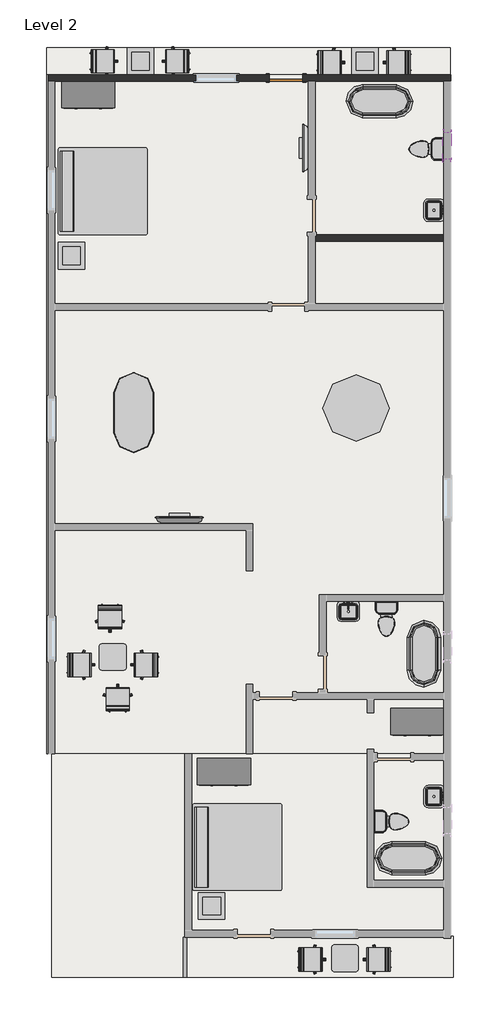
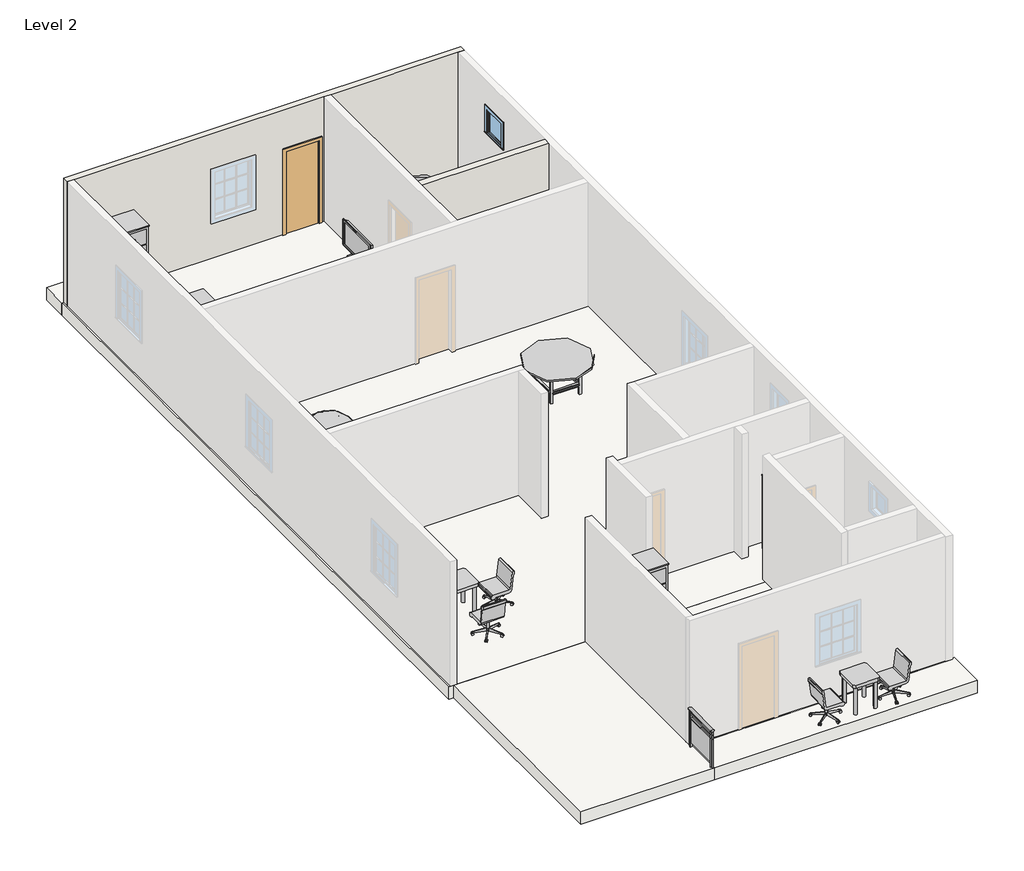
# One storey, part 2 of 2: 25 furniture elements, 9 flow terminals, 5 slabs, 2 walls, 1 door, 1 railing, 1 window.
"""IFC4 building model written with IfcOpenShell, lengths in millimetres."""

from ifc_helpers import new_model, si_unit, point, frame, origin, place, context, project, spatial, polyline, ellipse_curve, trimmed, outline, extrude, faceted_brep, transform, mapped, element, save
from ifc_brep_helpers import plane_surface, extruded_surface, advanced_brep
from components import door_255cab33, flow_terminal_62a433f7, toilet_domestic_3d_toilet_domestic_3d_f7549cf7, toilet_domestic_3d_toilet_domestic_3d_183bbd19, flow_terminal_b374fae2, furniture_1fc5af50, chair_task_chair_task_b7f3823b, furniture_9fa109b2, furniture_7a3aaa4f, furniture_b5c51a22, furniture_2c34a4f9, furniture_bbcc68ce, furniture_bcf351fa, window_3d781103

model = new_model("IFC4")

# Units and contexts
model_context = context("Model", 3, world=origin())
ifc_project = project(units=[si_unit("LENGTHUNIT", "METRE", prefix="MILLI")], contexts=[model_context])

# Site, building, storey
site = spatial("IfcSite", under=ifc_project)
building = spatial("IfcBuilding", under=site)
storey = spatial("IfcBuildingStorey", under=building, Name="Level 2", Elevation=3048.0)

# Door
placement = place(None, origin())
door_shape = door_255cab33(model_context)
element("IfcDoor", 1, ObjectType="Single-Flush : 30\" x 80\"", at=placement, inside=storey, context=model_context, shape_type="MappedRepresentation", body=[
    mapped(door_shape, transform((-7116.1873398, 12389.5549175, 3048.0), x_axis=(1.0, 0.0, 0.0), y_axis=(0.0, 1.0, 0.0), z_axis=(0.0, 0.0, 1.0))),
])

# Flow terminals
flow_terminal_shape = flow_terminal_62a433f7(model_context)
element("IfcFlowTerminal", 2, ObjectType="Sink Vanity-Square : 20\" x 18\"", at=placement, inside=storey, context=model_context, shape_type="MappedRepresentation", body=[
    mapped(flow_terminal_shape, transform((-3689.5327409, -4015.8558419, 3352.8), x_axis=(0.0, -0.9999999999999997, 0.0), y_axis=(0.9999999999999997, 0.0, 0.0), z_axis=(0.0, 0.0, 1.0))),
])
element("IfcFlowTerminal", 3, ObjectType="Sink Vanity-Square : 20\" x 18\"", at=placement, inside=storey, context=model_context, shape_type="MappedRepresentation", body=[
    mapped(flow_terminal_shape, transform((-5709.4765804, 246.0095164, 3048.0), x_axis=(1.0, 0.0, 0.0), y_axis=(0.0, 1.0, 0.0), z_axis=(0.0, 0.0, 1.0))),
])
element("IfcFlowTerminal", 4, ObjectType="Sink Vanity-Square : 20\" x 18\"", at=placement, inside=storey, context=model_context, shape_type="MappedRepresentation", body=[
    mapped(flow_terminal_shape, transform((-3689.5327409, 9382.6441581, 3352.8), x_axis=(0.0, -1.0000000000000004, 0.0), y_axis=(1.0000000000000004, 0.0, 0.0), z_axis=(0.0, 0.0, 1.0))),
])
toilet_domestic_3d_toilet_domestic_3d_shape = toilet_domestic_3d_toilet_domestic_3d_f7549cf7(model_context)
toilet_domestic_3d_toilet_domestic_3d_2_shape = toilet_domestic_3d_toilet_domestic_3d_183bbd19(model_context)
element("IfcFlowTerminal", 5, ObjectType="Toilet-Domestic-3D : Toilet-Domestic-3D", at=placement, inside=storey, context=model_context, shape_type="MappedRepresentation", body=[
    mapped(toilet_domestic_3d_toilet_domestic_3d_shape, transform((-4004.0833671, 10763.9549175, 3048.0), x_axis=(0.0, -1.0000000000000004, 0.0), y_axis=(1.0000000000000004, 0.0, 0.0), z_axis=(0.0, 0.0, 1.0))),
    mapped(toilet_domestic_3d_toilet_domestic_3d_2_shape, transform((-4004.0833671, 10763.9549175, 3048.0), x_axis=(0.0, -1.0000000000000004, 0.0), y_axis=(1.0000000000000004, 0.0, 0.0), z_axis=(0.0, 0.0, 1.0))),
])
element("IfcFlowTerminal", 6, ObjectType="Toilet-Domestic-3D : Toilet-Domestic-3D", at=placement, inside=storey, context=model_context, shape_type="MappedRepresentation", body=[
    mapped(toilet_domestic_3d_toilet_domestic_3d_shape, transform((-4614.8913124, -4603.0450825, 3048.0), x_axis=(0.0, 1.0, 0.0), y_axis=(-1.0, 0.0, 0.0), z_axis=(0.0, 0.0, 1.0))),
    mapped(toilet_domestic_3d_toilet_domestic_3d_2_shape, transform((-4614.8913124, -4603.0450825, 3048.0), x_axis=(0.0, 1.0, 0.0), y_axis=(-1.0, 0.0, 0.0), z_axis=(0.0, 0.0, 1.0))),
])
element("IfcFlowTerminal", 7, ObjectType="Toilet-Domestic-3D : Toilet-Domestic-3D", at=placement, inside=storey, context=model_context, shape_type="MappedRepresentation", body=[
    mapped(toilet_domestic_3d_toilet_domestic_3d_shape, transform((-4823.8668352, -68.5411098, 3048.0), x_axis=(1.0, 0.0, 0.0), y_axis=(0.0, 1.0, 0.0), z_axis=(0.0, 0.0, 1.0))),
    mapped(toilet_domestic_3d_toilet_domestic_3d_2_shape, transform((-4823.8668352, -68.5411098, 3048.0), x_axis=(1.0, 0.0, 0.0), y_axis=(0.0, 1.0, 0.0), z_axis=(0.0, 0.0, 1.0))),
])
flow_terminal_2_shape = flow_terminal_b374fae2(model_context)
element("IfcFlowTerminal", 8, ObjectType="Tub-Free Standing-3D : 30\" x 60\"", at=placement, inside=storey, context=model_context, shape_type="MappedRepresentation", body=[
    mapped(flow_terminal_2_shape, transform((-4322.1873398, -5441.2450825, 3048.0), x_axis=(0.0, -0.9999999999999998, 0.0), y_axis=(0.9999999999999998, 0.0, 0.0), z_axis=(0.0, 0.0, 1.0))),
])
element("IfcFlowTerminal", 9, ObjectType="Tub-Free Standing-3D : 30\" x 60\"", at=placement, inside=storey, context=model_context, shape_type="MappedRepresentation", body=[
    mapped(flow_terminal_2_shape, transform((-3966.5873398, -767.6450825, 3048.0), x_axis=(1.0, 0.0, 0.0), y_axis=(0.0, 1.0, 0.0), z_axis=(0.0, 0.0, 1.0))),
])
element("IfcFlowTerminal", 10, ObjectType="Tub-Free Standing-3D : 30\" x 60\"", at=placement, inside=storey, context=model_context, shape_type="MappedRepresentation", body=[
    mapped(flow_terminal_2_shape, transform((-4982.5873398, 11856.1549175, 3048.0), x_axis=(0.0, 1.0, 0.0), y_axis=(-1.0, 0.0, 0.0), z_axis=(0.0, 0.0, 1.0))),
])

# Furniture
furniture_shape = furniture_1fc5af50(model_context)
element("IfcFurniture", 11, ObjectType="Bed-Standard : King 78\" x 80\"", at=placement, inside=storey, context=model_context, shape_type="MappedRepresentation", body=[
    mapped(furniture_shape, transform((-8279.3824218, -5458.733607, 3048.0), x_axis=(0.0, 1.0000000000000002, 0.0), y_axis=(-1.0000000000000002, 0.0, 0.0), z_axis=(0.0, 0.0, 1.0))),
])
element("IfcFurniture", 12, ObjectType="Bed-Standard : King 78\" x 80\"", at=placement, inside=storey, context=model_context, shape_type="MappedRepresentation", body=[
    mapped(furniture_shape, transform((-11352.7824218, 9527.266393, 3048.0), x_axis=(0.0, 1.0000000000000002, 0.0), y_axis=(-1.0000000000000002, 0.0, 0.0), z_axis=(0.0, 0.0, 1.0))),
])
chair_task_chair_task_shape = chair_task_chair_task_b7f3823b(model_context)
element("IfcFurniture", 13, ObjectType="Chair-Task : Chair-Task", at=placement, inside=storey, context=model_context, shape_type="MappedRepresentation", body=[
    mapped(chair_task_chair_task_shape, transform((-9586.4414382, 12629.5640979, 3048.0), x_axis=(0.0, 1.0000000000000009, 0.0), y_axis=(-1.0000000000000009, 0.0, 0.0), z_axis=(0.0, 0.0, 1.0))),
])
element("IfcFurniture", 14, ObjectType="Chair-Task : Chair-Task", at=placement, inside=storey, context=model_context, shape_type="MappedRepresentation", body=[
    mapped(chair_task_chair_task_shape, transform((-6144.5332414, 12886.1457372, 3048.0), x_axis=(0.0, -1.0000000000000007, 0.0), y_axis=(1.0000000000000007, 0.0, 0.0), z_axis=(0.0, 0.0, 1.0))),
])
element("IfcFurniture", 15, ObjectType="Chair-Task : Chair-Task", at=placement, inside=storey, context=model_context, shape_type="MappedRepresentation", body=[
    mapped(chair_task_chair_task_shape, transform((-4531.8414382, 12604.1640979, 3048.0), x_axis=(0.0, 1.0000000000000007, 0.0), y_axis=(-1.0000000000000007, 0.0, 0.0), z_axis=(0.0, 0.0, 1.0))),
])
element("IfcFurniture", 16, ObjectType="Chair-Task : Chair-Task", at=placement, inside=storey, context=model_context, shape_type="MappedRepresentation", body=[
    mapped(chair_task_chair_task_shape, transform((-11326.1332414, 12911.5457372, 3048.0), x_axis=(0.0, -1.0000000000000009, 0.0), y_axis=(1.0000000000000009, 0.0, 0.0), z_axis=(0.0, 0.0, 1.0))),
])
element("IfcFurniture", 17, ObjectType="Chair-Task : Chair-Task", at=placement, inside=storey, context=model_context, shape_type="MappedRepresentation", body=[
    mapped(chair_task_chair_task_shape, transform((-4989.0414382, -7893.6359021, 3048.0), x_axis=(0.0, 1.0000000000000009, 0.0), y_axis=(-1.0000000000000009, 0.0, 0.0), z_axis=(0.0, 0.0, 1.0))),
])
element("IfcFurniture", 18, ObjectType="Chair-Task : Chair-Task", at=placement, inside=storey, context=model_context, shape_type="MappedRepresentation", body=[
    mapped(chair_task_chair_task_shape, transform((-6576.3332414, -7611.6542628, 3048.0), x_axis=(0.0, -1.0000000000000004, 0.0), y_axis=(1.0000000000000004, 0.0, 0.0), z_axis=(0.0, 0.0, 1.0))),
])
element("IfcFurniture", 19, ObjectType="Chair-Task : Chair-Task", at=placement, inside=storey, context=model_context, shape_type="MappedRepresentation", body=[
    mapped(chair_task_chair_task_shape, transform((-11105.2781595, -1827.9909841, 3048.0), x_axis=(1.0, 0.0, 0.0), y_axis=(0.0, 1.0, 0.0), z_axis=(0.0, 0.0, 1.0))),
])
element("IfcFurniture", 20, ObjectType="Chair-Task : Chair-Task", at=placement, inside=storey, context=model_context, shape_type="MappedRepresentation", body=[
    mapped(chair_task_chair_task_shape, transform((-11001.0965201, 89.5008192, 3048.0), x_axis=(-1.0000000000000004, 0.0, 0.0), y_axis=(0.0, -1.0000000000000004, 0.0), z_axis=(0.0, 0.0, 1.0))),
])
element("IfcFurniture", 21, ObjectType="Chair-Task : Chair-Task", at=placement, inside=storey, context=model_context, shape_type="MappedRepresentation", body=[
    mapped(chair_task_chair_task_shape, transform((-10297.6414382, -1162.6359021, 3048.0), x_axis=(0.0, 1.000000000000001, 0.0), y_axis=(-1.000000000000001, 0.0, 0.0), z_axis=(0.0, 0.0, 1.0))),
])
element("IfcFurniture", 22, ObjectType="Chair-Task : Chair-Task", at=placement, inside=storey, context=model_context, shape_type="MappedRepresentation", body=[
    mapped(chair_task_chair_task_shape, transform((-11853.1832414, -880.6542628, 3048.0), x_axis=(0.0, -1.0000000000000007, 0.0), y_axis=(1.0000000000000007, 0.0, 0.0), z_axis=(0.0, 0.0, 1.0))),
])
furniture_2_shape = furniture_9fa109b2(model_context)
element("IfcFurniture", 23, ObjectType="Dresser : 48\" x 72\" x 24\"", at=placement, inside=storey, context=model_context, shape_type="MappedRepresentation", body=[
    mapped(furniture_2_shape, transform((-8269.39408, -3096.8821284, 3048.0), x_axis=(1.0, 0.0, 0.0), y_axis=(0.0, 1.0, 0.0), z_axis=(0.0, 0.0, 1.0))),
])
element("IfcFurniture", 24, ObjectType="Dresser : 48\" x 72\" x 24\"", at=placement, inside=storey, context=model_context, shape_type="MappedRepresentation", body=[
    mapped(furniture_2_shape, transform((-11368.19408, 12371.7178716, 3048.0), x_axis=(1.0, 0.0, 0.0), y_axis=(0.0, 1.0, 0.0), z_axis=(0.0, 0.0, 1.0))),
])
element("IfcFurniture", 25, ObjectType="Dresser : 48\" x 72\" x 24\"", at=placement, inside=storey, context=model_context, shape_type="MappedRepresentation", body=[
    mapped(furniture_2_shape, transform((-3849.79408, -1953.8821284, 3048.0), x_axis=(1.0, 0.0, 0.0), y_axis=(0.0, 1.0, 0.0), z_axis=(0.0, 0.0, 1.0))),
])
furniture_3_shape = furniture_7a3aaa4f(model_context)
element("IfcFurniture", 26, ObjectType="TV - Flat Screen : 42\"", at=placement, inside=storey, context=model_context, shape_type="MappedRepresentation", body=[
    mapped(furniture_3_shape, transform((-6666.7259634, 10785.4104034, 3048.0), x_axis=(0.0, -1.0000000000000002, 0.0), y_axis=(1.0000000000000002, 0.0, 0.0), z_axis=(0.0, 0.0, 1.0))),
])
element("IfcFurniture", 27, ObjectType="TV - Flat Screen : 42\"", at=placement, inside=storey, context=model_context, shape_type="MappedRepresentation", body=[
    mapped(furniture_3_shape, transform((-9558.5318539, 2288.0935412, 3962.4), x_axis=(-1.000000000000001, 0.0, 0.0), y_axis=(0.0, -1.000000000000001, 0.0), z_axis=(0.0, 0.0, 1.0))),
])
furniture_4_shape = furniture_b5c51a22(model_context)
element("IfcFurniture", 28, ObjectType="Table-Coffee : 24\" x 24\" x 24\"", at=placement, inside=storey, context=model_context, shape_type="MappedRepresentation", body=[
    mapped(furniture_4_shape, transform((-10461.8531065, 12675.3438397, 3048.0), x_axis=(1.0, 0.0, 0.0), y_axis=(0.0, 1.0, 0.0), z_axis=(0.0, 0.0, 1.0))),
])
element("IfcFurniture", 29, ObjectType="Table-Coffee : 24\" x 24\" x 24\"", at=placement, inside=storey, context=model_context, shape_type="MappedRepresentation", body=[
    mapped(furniture_4_shape, transform((-5331.0531065, 12675.3438397, 3048.0), x_axis=(1.0, 0.0, 0.0), y_axis=(0.0, 1.0, 0.0), z_axis=(0.0, 0.0, 1.0))),
])
element("IfcFurniture", 30, ObjectType="Table-Coffee : 24\" x 24\" x 24\"", at=placement, inside=storey, context=model_context, shape_type="MappedRepresentation", body=[
    mapped(furniture_4_shape, transform((-8836.2531065, -6628.6561603, 3048.0), x_axis=(1.0, 0.0, 0.0), y_axis=(0.0, 1.0, 0.0), z_axis=(0.0, 0.0, 1.0))),
])
element("IfcFurniture", 31, ObjectType="Table-Coffee : 24\" x 24\" x 24\"", at=placement, inside=storey, context=model_context, shape_type="MappedRepresentation", body=[
    mapped(furniture_4_shape, transform((-12036.6531065, 8230.3438397, 3048.0), x_axis=(1.0, 0.0, 0.0), y_axis=(0.0, 1.0, 0.0), z_axis=(0.0, 0.0, 1.0))),
])
furniture_5_shape = furniture_2c34a4f9(model_context)
element("IfcFurniture", 32, ObjectType="Table-Dining Oval : 36\" x 72\"", at=placement, inside=storey, context=model_context, shape_type="MappedRepresentation", body=[
    mapped(furniture_5_shape, transform((-10954.0857004, 5145.9745897, 3048.0), x_axis=(0.0, 1.0000000000000002, 0.0), y_axis=(-1.0000000000000002, 0.0, 0.0), z_axis=(0.0, 0.0, 1.0))),
])
furniture_6_shape = furniture_bbcc68ce(model_context)
element("IfcFurniture", 33, ObjectType="Table-Dining Round w Chairs : 60\" Diameter", at=placement, inside=storey, context=model_context, shape_type="MappedRepresentation", body=[
    mapped(furniture_6_shape, transform((-5619.669307, 5030.6336061, 3048.0), x_axis=(1.0, 0.0, 0.0), y_axis=(0.0, 1.0, 0.0), z_axis=(0.0, 0.0, 1.0))),
])
furniture_7_shape = furniture_bcf351fa(model_context)
element("IfcFurniture", 34, ObjectType="Table-End : 24\" x 24\"", at=placement, inside=storey, context=model_context, shape_type="MappedRepresentation", body=[
    mapped(furniture_7_shape, transform((-6078.5209701, -7879.6450825, 3048.0), x_axis=(1.0, 0.0, 0.0), y_axis=(0.0, 1.0, 0.0), z_axis=(0.0, 0.0, 1.0))),
])
element("IfcFurniture", 35, ObjectType="Table-End : 24\" x 24\"", at=placement, inside=storey, context=model_context, shape_type="MappedRepresentation", body=[
    mapped(furniture_7_shape, transform((-11387.1209701, -996.2450825, 3048.0), x_axis=(1.0, 0.0, 0.0), y_axis=(0.0, 1.0, 0.0), z_axis=(0.0, 0.0, 1.0))),
])

# Railing
element("IfcRailing", 36, ObjectType="Glass Panel - Bottom Fill", at=placement, inside=storey, context=model_context, shape_type="SolidModel", body=[
    advanced_brep(
    [(-9389.4873398, -7244.6450825, 3962.4), (-9465.6873398, -7244.6450825, 3962.4), (-9389.4873398, -8159.0450825, 3962.4), (-9465.6873398, -8159.0450825, 3962.4)],
    [
        (0, 1, ellipse_curve(frame((-9427.5873398, -7244.6450825, 3962.4), z_axis=(0.0, 1.0, 0.0), x_axis=(-1.0, 0.0, 0.0)), 38.1, 28.575)),
        (1, 0, ellipse_curve(frame((-9427.5873398, -7244.6450825, 3962.4), z_axis=(0.0, 1.0, 0.0), x_axis=(-1.0, 0.0, 0.0)), 38.1, 28.575)),
        (2, 3, ellipse_curve(frame((-9427.5873398, -8159.0450825, 3962.4), z_axis=(0.0, -1.0, 0.0), x_axis=(-1.0, 0.0, 0.0)), 38.1, 28.575)),
        (3, 2, ellipse_curve(frame((-9427.5873398, -8159.0450825, 3962.4), z_axis=(0.0, -1.0, 0.0), x_axis=(-1.0, 0.0, 0.0)), 38.1, 28.575)),
        (0, 2),
        (3, 1),
    ],
    [
        plane_surface(frame((-9427.5873398, -7244.6450825, 3962.4), z_axis=(0.0, 1.0, 0.0), x_axis=(0.0, 0.0, -1.0))),
        plane_surface(frame((-9427.5873398, -8159.0450825, 3962.4), z_axis=(0.0, -1.0, 0.0), x_axis=(0.0, 0.0, -1.0))),
        extruded_surface(trimmed(ellipse_curve(frame((-9427.5873398, -8159.0450825, 3962.4), z_axis=(0.0, 1.0, 0.0), x_axis=(-1.0, 0.0, 0.0)), 38.1, 28.575), [point((-9389.4873398, -8159.0450825, 3962.4))], [point((-9465.6873398, -8159.0450825, 3962.4))], True, "CARTESIAN"), (0.0, 914.3999999999996, 0.0), 914.3999999999996),
        extruded_surface(trimmed(ellipse_curve(frame((-9427.5873398, -8159.0450825, 3962.4), z_axis=(0.0, 1.0, 0.0), x_axis=(-1.0, 0.0, 0.0)), 38.1, 28.575), [point((-9465.6873398, -8159.0450825, 3962.4))], [point((-9389.4873398, -8159.0450825, 3962.4))], True, "CARTESIAN"), (0.0, 914.3999999999996, 0.0), 914.3999999999996),
    ],
    [
        (0, [[1, 2]]),
        (1, [[3, 4]]),
        (2, [[-1, 5, -4, 6]]),
        (3, [[-2, -6, -3, -5]]),
    ],
),
    extrude(outline(polyline([(-9440.2873398, -7244.6450825), (-9414.8873398, -7244.6450825), (-9414.8873398, -8159.0450825), (-9440.2873398, -8159.0450825), (-9440.2873398, -7244.6450825)])), frame((0.0, 0.0, 3848.1), z_axis=(0.0, 0.0, 1.0), x_axis=(1.0, 0.0, 0.0)), (0.0, 0.0, 1.0), 25.4),
    extrude(outline(polyline([(-9440.2873398, -7244.6450825), (-9414.8873398, -7244.6450825), (-9414.8873398, -8159.0450825), (-9440.2873398, -8159.0450825), (-9440.2873398, -7244.6450825)])), frame((0.0, 0.0, 3746.5), z_axis=(0.0, 0.0, 1.0), x_axis=(1.0, 0.0, 0.0)), (0.0, 0.0, 1.0), 25.4),
    extrude(outline(polyline([(-9452.9873398, -8101.8950825), (-9402.1873398, -8101.8950825), (-9402.1873398, -8114.5950825), (-9452.9873398, -8114.5950825), (-9452.9873398, -8101.8950825)])), frame((0.0, 0.0, 3048.0), z_axis=(0.0, 0.0, 1.0), x_axis=(1.0, 0.0, 0.0)), (0.0, 0.0, 1.0), 885.6788223),
    extrude(outline(polyline([(-9421.0521828, -7295.4450825), (-9421.0521828, -8108.2450825), (-9427.4021828, -8108.2450825), (-9427.4021828, -7295.4450825), (-9421.0521828, -7295.4450825)])), frame((0.0, 0.0, 3149.6), z_axis=(0.0, 0.0, 1.0), x_axis=(1.0, 0.0, 0.0)), (0.0, 0.0, 1.0), 596.9),
    extrude(outline(polyline([(-9452.9873398, -7289.0950825), (-9402.1873398, -7289.0950825), (-9402.1873398, -7301.7950825), (-9452.9873398, -7301.7950825), (-9452.9873398, -7289.0950825)])), frame((0.0, 0.0, 3048.0), z_axis=(0.0, 0.0, 1.0), x_axis=(1.0, 0.0, 0.0)), (0.0, 0.0, 1.0), 885.6788223),
    extrude(outline(polyline([(-9437.1123398, -8146.3450825), (-9418.0623398, -8146.3450825), (-9418.0623398, -8165.3950825), (-9437.1123398, -8165.3950825), (-9437.1123398, -8146.3450825)])), frame((0.0, 0.0, 3048.0), z_axis=(0.0, 0.0, 1.0), x_axis=(1.0, 0.0, 0.0)), (0.0, 0.0, 1.0), 885.6788223),
    extrude(outline(polyline([(-9437.1123398, -7238.2950825), (-9418.0623398, -7238.2950825), (-9418.0623398, -7257.3450825), (-9437.1123398, -7257.3450825), (-9437.1123398, -7238.2950825)])), frame((0.0, 0.0, 3048.0), z_axis=(0.0, 0.0, 1.0), x_axis=(1.0, 0.0, 0.0)), (0.0, 0.0, 1.0), 885.6788223),
])

# Slabs
element("IfcSlab", 37, ObjectType="Generic - 12\"", at=placement, inside=storey, context=model_context, shape_type="SweptSolid", body=[
    extrude(outline(polyline([(-9388.9070436, -3053.6450825), (-9388.9070436, -8159.0450825), (-12475.5873398, -8159.0450825), (-12475.5873398, -3053.6450825), (-9388.9070436, -3053.6450825)])), frame((0.0, 0.0, 2743.2), z_axis=(0.0, 0.0, 1.0), x_axis=(1.0, 0.0, 0.0)), (0.0, 0.0, 1.0), 304.8),
])
element("IfcSlab", 38, ObjectType="Generic - 12\"", at=placement, inside=storey, context=model_context, shape_type="SweptSolid", body=[
    extrude(outline(polyline([(-3292.9070436, -8159.0450825), (-9388.9070436, -8159.0450825), (-9388.9070436, -7219.2450825), (-3292.9070436, -7219.2450825), (-3292.9070436, -8159.0450825)])), frame((0.0, 0.0, 2743.2), z_axis=(0.0, 0.0, 1.0), x_axis=(1.0, 0.0, 0.0)), (0.0, 0.0, 1.0), 304.8),
])
element("IfcSlab", 39, ObjectType="Generic - 12\"", at=placement, inside=storey, context=model_context, shape_type="SweptSolid", body=[
    extrude(outline(polyline([(-3369.6873398, 12465.7549175), (-12589.8873398, 12465.7549175), (-12589.8873398, 13081.7049175), (-3369.6873398, 13081.7049175), (-3369.6873398, 12465.7549175)])), frame((0.0, 0.0, 2743.2), z_axis=(0.0, 0.0, 1.0), x_axis=(1.0, 0.0, 0.0)), (0.0, 0.0, 1.0), 304.8),
])
element("IfcSlab", 40, ObjectType="Generic - 12\"", at=placement, inside=storey, context=model_context, shape_type="SweptSolid", body=[
    extrude(outline(polyline([(-3509.3873398, 12459.4049175), (-3509.3873398, -3053.6450825), (-12590.467636, -3053.6450825), (-12590.467636, 12459.4049175), (-3509.3873398, 12459.4049175)])), frame((0.0, 0.0, 2743.2), z_axis=(0.0, 0.0, 1.0), x_axis=(1.0, 0.0, 0.0)), (0.0, 0.0, 1.0), 304.8),
])
element("IfcSlab", 41, ObjectType="Generic - 12\"", at=placement, inside=storey, context=model_context, shape_type="SweptSolid", body=[
    extrude(outline(polyline([(-3433.1873398, -3053.6450825), (-3433.1873398, -7270.0450825), (-9275.1873398, -7270.0450825), (-9275.1873398, -3053.6450825), (-3433.1873398, -3053.6450825)])), frame((0.0, 0.0, 2743.2), z_axis=(0.0, 0.0, 1.0), x_axis=(1.0, 0.0, 0.0)), (0.0, 0.0, 1.0), 304.8),
])

# Walls
element("IfcWall", 42, ObjectType="Generic - 8\"", at=placement, inside=storey, context=model_context, shape_type="Brep", body=[
    faceted_brep([(-6735.1873398, 12313.3549175, 5080.0), (-6735.1873398, 12313.3549175, 3048.0), (-6608.1873398, 12313.3549175, 3048.0), (-6455.7873398, 12313.3549175, 3048.0), (-3509.3873398, 12313.3549175, 3048.0), (-3356.9873398, 12313.3549175, 3048.0), (-3356.9873398, 12313.3549175, 6096.0), (-3509.3873398, 12313.3549175, 6096.0), (-6455.7873398, 12313.3549175, 6096.0), (-6608.1873398, 12313.3549175, 6096.0), (-12399.3873398, 12313.3549175, 6096.0), (-12551.7873398, 12313.3549175, 6096.0), (-12551.7873398, 12313.3549175, 3048.0), (-12399.3873398, 12313.3549175, 3048.0), (-7497.1873398, 12313.3549175, 3048.0), (-7497.1873398, 12313.3549175, 5080.0), (-8259.1873398, 12313.3549175, 5181.6), (-8259.1873398, 12313.3549175, 3962.4), (-9173.5873398, 12313.3549175, 3962.4), (-9173.5873398, 12313.3549175, 5181.6), (-3356.9873398, 12465.7549175, 3048.0), (-6735.1873398, 12465.7549175, 3048.0), (-6735.1873398, 12465.7549175, 5080.0), (-7497.1873398, 12465.7549175, 5080.0), (-7497.1873398, 12465.7549175, 3048.0), (-12551.7873398, 12465.7549175, 3048.0), (-12551.7873398, 12465.7549175, 6096.0), (-3356.9873398, 12465.7549175, 6096.0), (-8259.1873398, 12465.7549175, 5181.6), (-9173.5873398, 12465.7549175, 5181.6), (-9173.5873398, 12465.7549175, 3962.4), (-8259.1873398, 12465.7549175, 3962.4)], [[[0, 1, 2, 3, 4, 5, 6, 7, 8, 9, 10, 11, 12, 13, 14, 15], [16, 17, 18, 19]], [[20, 21, 22, 23, 24, 25, 26, 27], [28, 29, 30, 31]], [[14, 13, 12, 25, 24]], [[5, 4, 3, 2, 1, 21, 20]], [[11, 10, 9, 8, 7, 6, 27, 26]], [[22, 21, 1, 0]], [[23, 22, 0, 15]], [[24, 23, 15, 14]], [[17, 16, 28, 31]], [[18, 17, 31, 30]], [[19, 18, 30, 29]], [[16, 19, 29, 28]], [[6, 5, 20, 27]], [[12, 11, 26, 25]]]),
])
element("IfcWall", 43, ObjectType="Generic - 8\"", at=placement, inside=storey, context=model_context, shape_type="SweptSolid", body=[
    extrude(outline(polyline([(-3509.3873398, 8655.7549175), (-6455.7873398, 8655.7549175), (-6455.7873398, 8808.1549175), (-3509.3873398, 8808.1549175), (-3509.3873398, 8655.7549175)])), frame((0.0, 0.0, 3048.0), z_axis=(0.0, 0.0, 1.0), x_axis=(1.0, 0.0, 0.0)), (0.0, 0.0, 1.0), 3048.0),
])

# Window
window_shape = window_3d781103(model_context)
element("IfcWindow", 44, ObjectType="Transom with Trim : 24\" x 24\"", at=placement, inside=storey, context=model_context, shape_type="MappedRepresentation", body=[
    mapped(window_shape, transform((-3433.1873398, 10878.2549175, 2667.0), x_axis=(0.0, 1.0, 0.0), y_axis=(-1.0, 0.0, 0.0), z_axis=(0.0, 0.0, 1.0))),
])

save(model, "model.ifc")

# Revit data of these elements
# Type "Single-Flush : 30\" x 80\""
#   Type Mark = "5"
#   Construction Type Id = "MDOOR"
#   Assembly Code = "C1020"
#   Analytic Construction = "Metal"
#   Thickness = 0' - 2"
#   Heat Transfer Coefficient (U) = 0.651978 BTU/(h·ft²·°F)
#   Height = 6' - 8"
#   Trim Projection Ext = 0' - 1"
#   Trim Projection Int = 0' - 1"
#   Trim Width = 0' - 3"
#   Width = 2' - 6"
#   Define Thermal Properties by = 1
#   Door Material = Door - Panel
#   Frame Material = Door - Frame
#   Visual Light Transmittance = 0
#   Solar Heat Gain Coefficient = 0
#   Function = (empty or 0)
#   Wall Closure = (empty or 0)
# Type "Sink Vanity-Square : 20\" x 18\""
#   Assembly Code = "D2010400"
#   Counter Height = 2' - 7"
#   Depth = 1' - 6"
#   Width = 1' - 8"
#   Basin Material = Porcelain, Linen
#   Faucet Material = Steel, Polished
#   Default Elevation = 0
# Type "Toilet-Domestic-3D : Toilet-Domestic-3D"
#   Assembly Code = "D2010110"
#   Toilet - Bowl/Basin Material = Porcelain, Linen
#   Toilet - Seat Material = Laminate, Linen, Matte
#   Default Elevation = 0
# Type "Tub-Free Standing-3D : 30\" x 60\""
#   Assembly Code = "D2010110"
#   Height = 1' - 6"
#   Length = 5' - 0"
#   Width = 2' - 6"
#   Tub Material = Porcelain, Ivory
#   Default Elevation = 0
# Type "Bed-Standard : King 78\" x 80\""
#   Assembly Code = "E2020200"
#   Length = 6' - 8"
#   Width = 6' - 6"
#   Leg Material = Steel, Chrome Plated
#   Mattress Material = Linen, White
#   Default Elevation = 0
# Type "Chair-Task : Chair-Task"
#   Assembly Code = "E2020200"
#   Base Material = Plastic, Opaque Black
#   Caster Material = Plastic, Opaque Black
#   Seat/Back Material = Textile - Slate Blue
#   Default Elevation = 0
# Type "Dresser : 48\" x 72\" x 24\""
#   Assembly Code = "E2020200"
#   Depth = 2' - 0"
#   Height = 6' - 0"
#   Width = 4' - 0"
#   Dresser Material = Laminate - Ivory, Glossy
#   Drawer Material = Laminate, Ivory, Matte
#   Knob Material = Cherry
#   Default Elevation = 0
# Type "TV - Flat Screen : 42\""
#   SinAng = 0' - 0.0193"
#   L = 3' - 0.71517"
#   H = 1' - 8.65418"
#   Thickness = 0' - 4.33071"
#   Diagonal = 3' - 6.12598"
#   CosAng = 0' - 0.03431"
#   Stand [instance default] = yes
#   Default Elevation = 0
# Type "Table-Coffee : 24\" x 24\" x 24\""
#   Assembly Code = "E2020200"
#   Height = 2' - 0"
#   Length = 2' - 0"
#   Width = 2' - 0"
#   Top Material = none
#   Frame Material = none
#   Default Elevation = 0
# Type "Table-Dining Oval : 36\" x 72\""
#   Assembly Code = "E2020200"
#   Length = 6' - 0"
#   Width = 3' - 0"
#   Base Material = Steel, Chrome Plated
#   Top Material = Glass - Clear, Grey
#   Default Elevation = 0
#   Description = (empty or 0)
# Type "Table-Dining Round w Chairs : 60\" Diameter"
#   Assembly Code = "E2020200"
#   Radius = 2' - 6"
#   Diameter = 5' - 0"
#   Height = 2' - 6"
#   Chairs = 6
#   Base Material = Pine
#   Top Material = Laminate, Linen, Matte
#   Default Elevation = 0
# Type "Table-End : 24\" x 24\""
#   Assembly Code = "E2020200"
#   Height = 2' - 6"
#   Length = 2' - 0"
#   Width = 2' - 0"
#   Base Material = Birch
#   Top Material = Laminate, Ivory, Matte
#   Default Elevation = 0
# Type "Glass Panel - Bottom Fill"
#   Assembly Code = "C2010400"
#   built-in parameter 1008612 = 0.0416667 (stored number, unit not read)
#   built-in parameter 1008611 = 0.0416667 (stored number, unit not read)
#   built-in parameter 1008609 = 0.333333 (stored number, unit not read)
#   built-in parameter 1008604 = 0.166667 (stored number, unit not read)
#   built-in parameter 1008603 = 0.166667 (stored number, unit not read)
#   Railing Height = 3' - 0"
#   built-in parameter 1008630 = 2
#   built-in parameter 1008610 = 2
#   built-in parameter 1008618 = Baluster - Square : 3/4"
# Type "Generic - 12\""
#   Assembly Code = "B1010"
#   Function = 0
#   Layers, outside or top first: 1' - 0" no material (function 1)
# Type "Generic - 8\""
#   Assembly Code = "B2010"
#   Layers, outside or top first: 0' - 6" "Brick, Common" (function 1)
# Type "Transom with Trim : 24\" x 24\""
#   Type Mark = "13"
#   Construction Type Id = "GSP4R"
#   Assembly Code = "B2020100"
#   Analytic Construction = "1/8 in Pilkington single glazing"
#   Visual Light Transmittance = 0.9
#   Solar Heat Gain Coefficient = 0.78
#   Heat Transfer Coefficient (U) = 0.6496 BTU/(h·ft²·°F)
#   Height = 2' - 0"
#   Default Sill Height = 7' - 1"
#   Trim Projection - Ext. = 0' - 0 1/2"
#   Trim Projection - Int. = 0' - 0 3/4"
#   Trim Width - Exterior = 0' - 3 1/2"
#   Trim Width - Interior = 0' - 3 1/2"
#   Width = 2' - 0"
#   Window Inset = 0' - 0 3/4"
#   Define Thermal Properties by = 1
#   Glass Pane Material = Glass
#   Sash Material = Sash
#   Trim Exterior Material = Trim
#   Trim Interior Material = Trim
#   Wall Closure = (empty or 0)
# Element 1 (IfcDoor, "Single-Flush : 30\" x 80\"")
#   Phase Created = New Construction
#   Materials on its faces: "Door - Frame", "Door - Panel"
# Element 2 (IfcFlowTerminal, "Sink Vanity-Square : 20\" x 18\"")
#   Mark = "14"
#   Phase Created = New Construction
#   Materials on its faces: "Porcelain, Linen", "Steel, Polished"
# Element 3 (IfcFlowTerminal, "Sink Vanity-Square : 20\" x 18\"")
#   Mark = "16"
#   Phase Created = New Construction
#   Materials on its faces: "Porcelain, Linen", "Steel, Polished"
# Element 4 (IfcFlowTerminal, "Sink Vanity-Square : 20\" x 18\"")
#   Mark = "18"
#   Phase Created = New Construction
#   Materials on its faces: "Porcelain, Linen", "Steel, Polished"
# Element 5 (IfcFlowTerminal, "Toilet-Domestic-3D : Toilet-Domestic-3D")
#   Mark = "9"
#   Phase Created = New Construction
#   Materials on its faces: "Porcelain, Linen", "Laminate, Linen, Matte"
# Element 6 (IfcFlowTerminal, "Toilet-Domestic-3D : Toilet-Domestic-3D")
#   Mark = "13"
#   Phase Created = New Construction
#   Materials on its faces: "Porcelain, Linen", "Laminate, Linen, Matte"
# Element 7 (IfcFlowTerminal, "Toilet-Domestic-3D : Toilet-Domestic-3D")
#   Mark = "17"
#   Phase Created = New Construction
#   Materials on its faces: "Porcelain, Linen", "Laminate, Linen, Matte"
# Element 8 (IfcFlowTerminal, "Tub-Free Standing-3D : 30\" x 60\"")
#   Mark = "11"
#   Phase Created = New Construction
#   Materials on its faces: "Porcelain, Ivory"
# Element 9 (IfcFlowTerminal, "Tub-Free Standing-3D : 30\" x 60\"")
#   Mark = "15"
#   Phase Created = New Construction
#   Materials on its faces: "Porcelain, Ivory"
# Element 10 (IfcFlowTerminal, "Tub-Free Standing-3D : 30\" x 60\"")
#   Mark = "19"
#   Phase Created = New Construction
#   Materials on its faces: "Porcelain, Ivory"
# Elements 11, 12 (IfcFurniture, "Bed-Standard : King 78\" x 80\"")
#   Phase Created = New Construction
#   Materials on its faces: "Linen, White", "Steel, Chrome Plated"
# Elements 13, 14, 15, 16, 17, 18, 19, 20, 21, 22 (IfcFurniture, "Chair-Task : Chair-Task")
#   Phase Created = New Construction
#   Materials on its faces: "Plastic, Opaque Black", "Textile - Slate Blue"
# Elements 23, 24, 25 (IfcFurniture, "Dresser : 48\" x 72\" x 24\"")
#   Phase Created = New Construction
#   Materials on its faces: "Laminate, Ivory, Matte", "Cherry", "Laminate - Ivory, Glossy"
# Elements 26, 27 (IfcFurniture, "TV - Flat Screen : 42\"")
#   Stand = yes
#   Phase Created = New Construction
#   Materials on its faces: "TV - Black", "TV - Glass", "TV - Screen"
# Elements 28, 29, 30, 31 (IfcFurniture, "Table-Coffee : 24\" x 24\" x 24\"")
#   Phase Created = New Construction
#   Materials on its faces: "Glass - Clear, Grey"
# Element 32 (IfcFurniture, "Table-Dining Oval : 36\" x 72\"")
#   Phase Created = New Construction
#   Materials on its faces: "Steel, Chrome Plated", "Glass - Clear, Grey"
# Element 33 (IfcFurniture, "Table-Dining Round w Chairs : 60\" Diameter")
#   Phase Created = New Construction
#   Materials on its faces: "Pine", "Laminate, Linen, Matte"
# Elements 34, 35 (IfcFurniture, "Table-End : 24\" x 24\"")
#   Phase Created = New Construction
#   Materials on its faces: "Laminate, Ivory, Matte", "Birch"
# Element 36 (IfcRailing, "Glass Panel - Bottom Fill")
#   Phase Created = New Construction
#   Materials on its faces: "Glass"
# Elements 37, 38, 39, 40, 41 (IfcSlab, "Generic - 12\"")
#   Height Offset From Level = 0' - 0"
#   Phase Created = New Construction
#   Materials on its faces: "Default Floor"
# Elements 42, 43 (IfcWall, "Generic - 8\"")
#   Top Offset = 0' - 0"
#   Base Offset = 0' - 0"
#   Unconnected Height = 10' - 0"
#   wall height = 10' - 0"
#   Phase Created = New Construction
#   Base Constraint = Level 2
#   Materials on its faces: "Brick, Common"
# Element 44 (IfcWindow, "Transom with Trim : 24\" x 24\"")
#   Mark = "21"
#   Phase Created = New Construction
#   Materials on its faces: "Sash", "Trim", "Glass"
# Materials
#   "Door - Panel": class "Wood", colour RGB 210 159 95, transparency 0
#   "Door - Frame": colour RGB 118 70 51, transparency 0
#   "Porcelain, Linen": class "Ceramic", colour RGB 249 239 230, transparency 0, Description = "Porcelain, linen", Cost = 0
#   "Steel, Polished": class "Metal", colour RGB 57 57 57, transparency 0, Description = "Polished steel", Cost = 0
#   "Laminate, Linen, Matte": class "Plastic", colour RGB 249 239 230, transparency 0, Description = "Plastic Laminate - Linen, Matte", Cost = 0
#   "Porcelain, Ivory": class "Ceramic", colour RGB 247 247 239, transparency 0, Description = "Porcelain, ivory", Cost = 0
#   "Steel, Chrome Plated": class "Metal", colour RGB 17 17 17, transparency 0, Description = "Chromiuim plated steel", Cost = 0
#   "Linen, White": class "Textile", colour RGB 247 247 239, transparency 0, Description = "Linen, white", Cost = 0
#   "Plastic, Opaque Black": class "Plastic", colour RGB 0 0 0, transparency 0.7, Description = "Plastic, generic, opaque black", Cost = 0
#   "Textile - Slate Blue": class "Fabric", colour RGB 98 102 118, transparency 0
#   "Laminate - Ivory, Glossy": colour RGB 247 247 239, transparency 0
#   "Laminate, Ivory, Matte": class "Plastic", colour RGB 247 247 239, transparency 0, Description = "Plastic Laminate - Ivory, Matte", Cost = 0
#   "Cherry": class "Wood", colour RGB 226 177 128, transparency 0, Description = "Prunus Serotina", Cost = 0
#   "Glass - Clear, Grey": class "Glass", colour RGB 252 255 255, transparency 0.64
#   "Pine": class "Wood", colour RGB 223 192 134, transparency 0, Description = "Pinus Echinata", Cost = 0
#   "Birch": class "Wood", colour RGB 224 178 126, transparency 0, Description = "Betula Alleghaniensis", Cost = 0
#   "Brick, Common": class "Masonry", colour RGB 170 98 104, transparency 0, Description = "Common brick", Cost = 0
#   "Glass": class "Glass", colour RGB 0 128 192, transparency 0.75, Description = "Soda Lime Glass", Cost = 0
#   "Sash": class "Wood", colour RGB 224 178 126, transparency 0
#   "Trim": class "Wood", colour RGB 224 178 126, transparency 0
#   "TV - Black": colour RGB 49 49 49, transparency 0
#   "TV - Glass": colour RGB 157 157 157, transparency 0.9
#   "TV - Screen": colour RGB 0 0 0, transparency 0
#   "Default Floor": colour RGB 128 128 128, transparency 0
